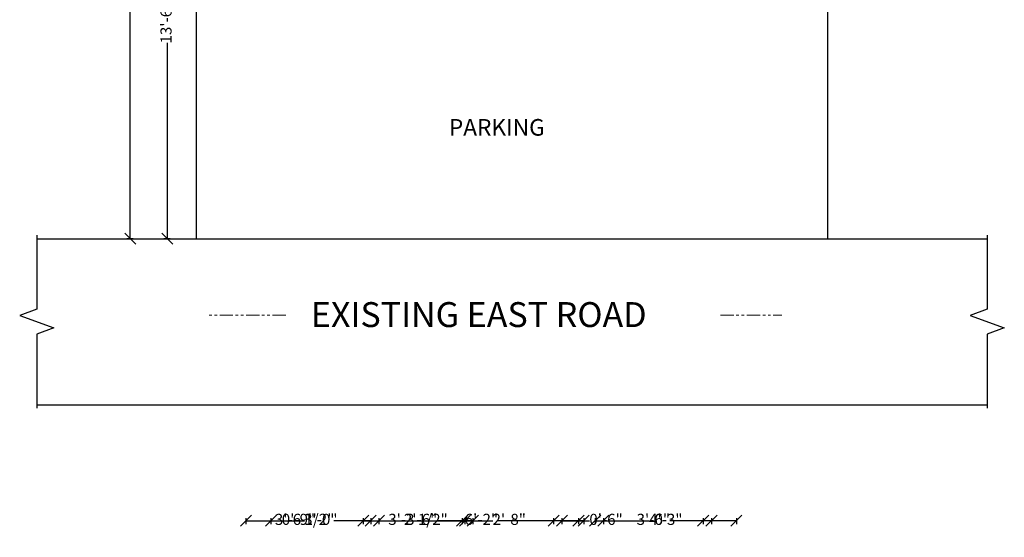
# Model space of a CAD drawing. Units: inches. Extents: x 2349 to 2798, y 397 to 1271.
# Tile 1 of 3: x 2396 to 2751, y 397 to 584. Entities that reach past the tile are written whole.
import ezdxf

# ---------------------------------------------------------------- set-up
doc = ezdxf.new("R2010")
doc.units = ezdxf.units.IN
doc.linetypes.add('PHANTOM2', pattern=[31.75, 15.875, -3.175, 3.175, -3.175, 3.175, -3.175])
for name, color, linetype, lineweight in [('A-ANNO-DIMS', 2, 'Continuous', 18), ('A-ANNO-TEXT', 7, 'Continuous', 18), ('A-AREA-IDEN', 7, 'Continuous', 18), ('C-PROP', 7, 'Continuous', 25), ('C-ROAD', 7, 'Continuous', 25), ('C-ROAD-CNTR', 7, 'PHANTOM2', 13)]:
    doc.layers.add(name, color=color, linetype=linetype, lineweight=lineweight)
doc.styles.get("Standard").update_dxf_attribs({"font": 'arial.ttf'})
doc.dimstyles.new('ISO-25', dxfattribs={"dimtxt": 4, "dimasz": 4, "dimexe": 1.25, "dimexo": 1, "dimtad": 0, "dimdec": 1, "dimlunit": 3, "dimtxsty": 'Standard', "dimblk": 'OBLIQUE', "dimcen": 2.5, "dimclrd": 1, "dimclrt": 3, "dimadec": 0, "dimazin": 0, "dimtfac": 1, "dimtdec": 1, "dimtmove": 0, "dimatfit": 3, "dimfxl": 1, "dimfxlon": 1, "dimarcsym": 0})

# ---------------------------------------------------------------- blocks, each defined once
blk = doc.blocks.new('_Oblique')
at = {"color": 0, "linetype": 'ByBlock', "lineweight": -2}
blk.add_line((-0.5, -0.5), (0.5, 0.5), dxfattribs=at)
blk = doc.blocks.new('*D9')
at = {"layer": 'A-ANNO-DIMS', "color": 0, "lineweight": -2, "transparency": 16777216}
for p, q in [((2450.39, 660.52), (2448.14, 660.52)), ((2449.39, 660.52), (2449.39, 589.82)), ((2449.39, 504.52), (2449.39, 575.21)), ((2450.39, 504.52), (2448.14, 504.52))]:
    blk.add_line(p, q, dxfattribs=at)
at = {"layer": 'Defpoints', "color": 0, "transparency": 16777216}
for p in [(2459.73, 660.52), (2449.39, 504.52), (2459.73, 504.52)]:
    blk.add_point(p, dxfattribs=at)
at = {"layer": 'A-ANNO-DIMS', "color": 0, "lineweight": -2, "transparency": 16777216, "xscale": 4, "yscale": 4, "zscale": 4}
for p, rotation in [((2449.39, 660.52), 90), ((2449.39, 504.52), 270)]:
    blk.add_blockref('_Oblique', p, dxfattribs=dict(at, rotation=rotation))
at = {"layer": 'A-ANNO-DIMS', "color": 0, "transparency": 16777216, "insert": (2449.39, 582.52), "char_height": 4, "attachment_point": 5, "rotation": 90}
blk.add_mtext('13\'-6"', dxfattribs=at)
blk = doc.blocks.new('*D10')
at = {"layer": 'A-ANNO-DIMS', "color": 0, "lineweight": -2, "transparency": 16777216}
for p, q in [((2436.96, 1224.52), (2434.71, 1224.52)), ((2435.96, 1224.52), (2435.96, 868.55)), ((2435.96, 504.52), (2435.96, 860.49)), ((2436.96, 504.52), (2434.71, 504.52))]:
    blk.add_line(p, q, dxfattribs=at)
at = {"layer": 'Defpoints', "color": 0, "transparency": 16777216}
for p in [(2459.73, 1224.52), (2435.96, 504.52), (2459.73, 504.52)]:
    blk.add_point(p, dxfattribs=at)
at = {"layer": 'A-ANNO-DIMS', "color": 0, "lineweight": -2, "transparency": 16777216, "xscale": 4, "yscale": 4, "zscale": 4}
for p, rotation in [((2435.96, 1224.52), 90), ((2435.96, 504.52), 270)]:
    blk.add_blockref('_Oblique', p, dxfattribs=dict(at, rotation=rotation))
at = {"layer": 'A-ANNO-DIMS', "color": 0, "transparency": 16777216, "insert": (2435.96, 864.52), "char_height": 4, "attachment_point": 5, "rotation": 90}
blk.add_mtext("60'", dxfattribs=at)
blk = doc.blocks.new('ROAD-BREAK')
blk.add_lwpolyline([(0, 0), (0, -26.75), (-6.18, -29), (6.18, -33.5), (0, -35.75), (0, -62.5)])
blk = doc.blocks.new('*D28')
at = {"layer": 'A-ANNO-DIMS', "color": 0, "lineweight": -2, "transparency": 16777216}
for p, q in [((2603.73, 403.67), (2603.73, 401.42)), ((2654.73, 403.67), (2654.73, 401.42))]:
    blk.add_line(p, q, dxfattribs=at)
at = {"layer": 'A-ANNO-DIMS', "color": 1, "lineweight": -2, "transparency": 16777216}
for p, q in [((2603.73, 402.67), (2623.21, 402.67)), ((2654.73, 402.67), (2635.25, 402.67))]:
    blk.add_line(p, q, dxfattribs=at)
at = {"layer": 'Defpoints', "color": 0, "transparency": 16777216}
for p in [(2603.73, 660.52), (2654.73, 660.52), (2654.73, 402.67)]:
    blk.add_point(p, dxfattribs=at)
at = {"layer": 'A-ANNO-DIMS', "color": 1, "lineweight": -2, "transparency": 16777216, "xscale": 4, "yscale": 4, "zscale": 4, "rotation": 180}
blk.add_blockref('_Oblique', (2603.73, 402.67), dxfattribs=at)
at = {"layer": 'A-ANNO-DIMS', "color": 1, "lineweight": -2, "transparency": 16777216, "xscale": 4, "yscale": 4, "zscale": 4}
blk.add_blockref('_Oblique', (2654.73, 402.67), dxfattribs=at)
at = {"layer": 'A-ANNO-DIMS', "color": 3, "transparency": 16777216, "insert": (2629.23, 402.67), "char_height": 4, "attachment_point": 5}
blk.add_mtext('4\'-3"', dxfattribs=at)
blk = doc.blocks.new('*D29')
at = {"layer": 'A-ANNO-DIMS', "color": 0, "lineweight": -2, "transparency": 16777216}
for p, q in [((2477.73, 403.67), (2477.73, 401.42)), ((2520.04, 403.67), (2520.04, 401.42))]:
    blk.add_line(p, q, dxfattribs=at)
at = {"layer": 'A-ANNO-DIMS', "color": 1, "lineweight": -2, "transparency": 16777216}
for p, q in [((2477.73, 402.67), (2488.28, 402.67)), ((2520.04, 402.67), (2509.48, 402.67))]:
    blk.add_line(p, q, dxfattribs=at)
at = {"layer": 'Defpoints', "color": 0, "transparency": 16777216}
for p in [(2477.73, 660.52), (2520.04, 660.52), (2520.04, 402.67)]:
    blk.add_point(p, dxfattribs=at)
at = {"layer": 'A-ANNO-DIMS', "color": 1, "lineweight": -2, "transparency": 16777216, "xscale": 4, "yscale": 4, "zscale": 4, "rotation": 180}
blk.add_blockref('_Oblique', (2477.73, 402.67), dxfattribs=at)
at = {"layer": 'A-ANNO-DIMS', "color": 1, "lineweight": -2, "transparency": 16777216, "xscale": 4, "yscale": 4, "zscale": 4}
blk.add_blockref('_Oblique', (2520.04, 402.67), dxfattribs=at)
at = {"layer": 'A-ANNO-DIMS', "color": 3, "transparency": 16777216, "insert": (2498.88, 402.67), "char_height": 4, "attachment_point": 5}
blk.add_mtext('3\'-6 1/2"', dxfattribs=at)
blk = doc.blocks.new('*D30')
at = {"layer": 'A-ANNO-DIMS', "color": 0, "lineweight": -2, "transparency": 16777216}
for p, q in [((2520.04, 403.67), (2520.04, 401.42)), ((2559.59, 403.67), (2559.59, 401.42))]:
    blk.add_line(p, q, dxfattribs=at)
at = {"layer": 'A-ANNO-DIMS', "color": 1, "lineweight": -2, "transparency": 16777216}
for p, q in [((2520.04, 402.67), (2529.21, 402.67)), ((2559.59, 402.67), (2550.42, 402.67))]:
    blk.add_line(p, q, dxfattribs=at)
at = {"layer": 'Defpoints', "color": 0, "transparency": 16777216}
for p in [(2520.04, 660.52), (2559.59, 660.52), (2559.59, 402.67)]:
    blk.add_point(p, dxfattribs=at)
at = {"layer": 'A-ANNO-DIMS', "color": 1, "lineweight": -2, "transparency": 16777216, "xscale": 4, "yscale": 4, "zscale": 4, "rotation": 180}
blk.add_blockref('_Oblique', (2520.04, 402.67), dxfattribs=at)
at = {"layer": 'A-ANNO-DIMS', "color": 1, "lineweight": -2, "transparency": 16777216, "xscale": 4, "yscale": 4, "zscale": 4}
blk.add_blockref('_Oblique', (2559.59, 402.67), dxfattribs=at)
at = {"layer": 'A-ANNO-DIMS', "color": 3, "transparency": 16777216, "insert": (2539.81, 402.67), "char_height": 4, "attachment_point": 5}
blk.add_mtext('3\'-3 1/2"', dxfattribs=at)
blk = doc.blocks.new('*D31')
at = {"layer": 'A-ANNO-DIMS', "color": 0, "lineweight": -2, "transparency": 16777216}
for p, q in [((2603.73, 403.67), (2603.73, 401.42)), ((2645.73, 403.67), (2645.73, 401.42))]:
    blk.add_line(p, q, dxfattribs=at)
at = {"layer": 'A-ANNO-DIMS', "color": 1, "lineweight": -2, "transparency": 16777216}
for p, q in [((2603.73, 402.67), (2618.79, 402.67)), ((2645.73, 402.67), (2630.67, 402.67))]:
    blk.add_line(p, q, dxfattribs=at)
at = {"layer": 'Defpoints', "color": 0, "transparency": 16777216}
for p in [(2603.73, 792.52), (2645.73, 792.52), (2645.73, 402.67)]:
    blk.add_point(p, dxfattribs=at)
at = {"layer": 'A-ANNO-DIMS', "color": 1, "lineweight": -2, "transparency": 16777216, "xscale": 4, "yscale": 4, "zscale": 4, "rotation": 180}
blk.add_blockref('_Oblique', (2603.73, 402.67), dxfattribs=at)
at = {"layer": 'A-ANNO-DIMS', "color": 1, "lineweight": -2, "transparency": 16777216, "xscale": 4, "yscale": 4, "zscale": 4}
blk.add_blockref('_Oblique', (2645.73, 402.67), dxfattribs=at)
at = {"layer": 'A-ANNO-DIMS', "color": 3, "transparency": 16777216, "insert": (2624.73, 402.67), "char_height": 4, "attachment_point": 5}
blk.add_mtext('3\'-6"', dxfattribs=at)
blk = doc.blocks.new('*D32')
at = {"layer": 'A-ANNO-DIMS', "color": 0, "lineweight": -2, "transparency": 16777216}
for p, q in [((2606.73, 403.67), (2606.73, 401.42)), ((2642.73, 403.67), (2642.73, 401.42))]:
    blk.add_line(p, q, dxfattribs=at)
at = {"layer": 'A-ANNO-DIMS', "color": 1, "lineweight": -2, "transparency": 16777216}
for p, q in [((2606.73, 402.67), (2618.79, 402.67)), ((2642.73, 402.67), (2630.67, 402.67))]:
    blk.add_line(p, q, dxfattribs=at)
at = {"layer": 'Defpoints', "color": 0, "transparency": 16777216}
for p in [(2606.73, 981.52), (2642.73, 981.52), (2642.73, 402.67)]:
    blk.add_point(p, dxfattribs=at)
at = {"layer": 'A-ANNO-DIMS', "color": 1, "lineweight": -2, "transparency": 16777216, "xscale": 4, "yscale": 4, "zscale": 4, "rotation": 180}
blk.add_blockref('_Oblique', (2606.73, 402.67), dxfattribs=at)
at = {"layer": 'A-ANNO-DIMS', "color": 1, "lineweight": -2, "transparency": 16777216, "xscale": 4, "yscale": 4, "zscale": 4}
blk.add_blockref('_Oblique', (2642.73, 402.67), dxfattribs=at)
at = {"layer": 'A-ANNO-DIMS', "color": 3, "transparency": 16777216, "insert": (2624.73, 402.67), "char_height": 4, "attachment_point": 5}
blk.add_mtext('3\'-0"', dxfattribs=at)
blk = doc.blocks.new('*D33')
at = {"layer": 'A-ANNO-DIMS', "color": 0, "lineweight": -2, "transparency": 16777216}
for p, q in [((2556.73, 403.67), (2556.73, 401.42)), ((2588.73, 403.67), (2588.73, 401.42))]:
    blk.add_line(p, q, dxfattribs=at)
at = {"layer": 'A-ANNO-DIMS', "color": 1, "lineweight": -2, "transparency": 16777216}
for p, q in [((2556.73, 402.67), (2566.76, 402.67)), ((2588.73, 402.67), (2578.71, 402.67))]:
    blk.add_line(p, q, dxfattribs=at)
at = {"layer": 'Defpoints', "color": 0, "transparency": 16777216}
for p in [(2556.73, 1143.52), (2588.73, 1143.52), (2588.73, 402.67)]:
    blk.add_point(p, dxfattribs=at)
at = {"layer": 'A-ANNO-DIMS', "color": 1, "lineweight": -2, "transparency": 16777216, "xscale": 4, "yscale": 4, "zscale": 4, "rotation": 180}
blk.add_blockref('_Oblique', (2556.73, 402.67), dxfattribs=at)
at = {"layer": 'A-ANNO-DIMS', "color": 1, "lineweight": -2, "transparency": 16777216, "xscale": 4, "yscale": 4, "zscale": 4}
blk.add_blockref('_Oblique', (2588.73, 402.67), dxfattribs=at)
at = {"layer": 'A-ANNO-DIMS', "color": 3, "transparency": 16777216, "insert": (2572.73, 402.67), "char_height": 4, "attachment_point": 5}
blk.add_mtext('2\'-8"', dxfattribs=at)
blk = doc.blocks.new('*D39')
at = {"layer": 'A-ANNO-DIMS', "color": 0, "lineweight": -2, "transparency": 16777216}
for p, q in [((2486.73, 403.67), (2486.73, 401.42)), ((2522.73, 403.67), (2522.73, 401.42))]:
    blk.add_line(p, q, dxfattribs=at)
at = {"layer": 'A-ANNO-DIMS', "color": 1, "lineweight": -2, "transparency": 16777216}
for p, q in [((2486.73, 402.67), (2498.79, 402.67)), ((2522.73, 402.67), (2510.67, 402.67))]:
    blk.add_line(p, q, dxfattribs=at)
at = {"layer": 'Defpoints', "color": 0, "transparency": 16777216}
for p in [(2486.73, 836.92), (2522.73, 836.92), (2522.73, 402.67)]:
    blk.add_point(p, dxfattribs=at)
at = {"layer": 'A-ANNO-DIMS', "color": 1, "lineweight": -2, "transparency": 16777216, "xscale": 4, "yscale": 4, "zscale": 4, "rotation": 180}
blk.add_blockref('_Oblique', (2486.73, 402.67), dxfattribs=at)
at = {"layer": 'A-ANNO-DIMS', "color": 1, "lineweight": -2, "transparency": 16777216, "xscale": 4, "yscale": 4, "zscale": 4}
blk.add_blockref('_Oblique', (2522.73, 402.67), dxfattribs=at)
at = {"layer": 'A-ANNO-DIMS', "color": 3, "transparency": 16777216, "insert": (2504.73, 402.67), "char_height": 4, "attachment_point": 5}
blk.add_mtext('3\'-0"', dxfattribs=at)
blk = doc.blocks.new('*D40')
at = {"layer": 'A-ANNO-DIMS', "color": 0, "lineweight": -2, "transparency": 16777216}
for p, q in [((2525.73, 403.67), (2525.73, 401.42)), ((2555.73, 403.67), (2555.73, 401.42))]:
    blk.add_line(p, q, dxfattribs=at)
at = {"layer": 'A-ANNO-DIMS', "color": 1, "lineweight": -2, "transparency": 16777216}
for p, q in [((2525.73, 402.67), (2534.76, 402.67)), ((2555.73, 402.67), (2546.71, 402.67))]:
    blk.add_line(p, q, dxfattribs=at)
at = {"layer": 'Defpoints', "color": 0, "transparency": 16777216}
for p in [(2555.73, 801.52), (2525.73, 795.52), (2555.73, 402.67)]:
    blk.add_point(p, dxfattribs=at)
at = {"layer": 'A-ANNO-DIMS', "color": 1, "lineweight": -2, "transparency": 16777216, "xscale": 4, "yscale": 4, "zscale": 4, "rotation": 180}
blk.add_blockref('_Oblique', (2525.73, 402.67), dxfattribs=at)
at = {"layer": 'A-ANNO-DIMS', "color": 1, "lineweight": -2, "transparency": 16777216, "xscale": 4, "yscale": 4, "zscale": 4}
blk.add_blockref('_Oblique', (2555.73, 402.67), dxfattribs=at)
at = {"layer": 'A-ANNO-DIMS', "color": 3, "transparency": 16777216, "insert": (2540.73, 402.67), "char_height": 4, "attachment_point": 5}
blk.add_mtext('2\'-6"', dxfattribs=at)
blk = doc.blocks.new('*D46')
at = {"layer": 'A-ANNO-DIMS', "color": 0, "lineweight": -2, "transparency": 16777216}
for p, q in [((2591.73, 403.67), (2591.73, 401.42)), ((2597.73, 403.67), (2597.73, 401.42))]:
    blk.add_line(p, q, dxfattribs=at)
at = {"layer": 'A-ANNO-DIMS', "color": 1, "lineweight": -2, "transparency": 16777216}
for p, q in [((2591.73, 402.67), (2597.73, 402.67)), ((2597.73, 402.67), (2601.73, 402.67))]:
    blk.add_line(p, q, dxfattribs=at)
at = {"layer": 'Defpoints', "color": 0, "transparency": 16777216}
for p in [(2591.73, 1206.52), (2597.73, 1206.52), (2597.73, 402.67)]:
    blk.add_point(p, dxfattribs=at)
at = {"layer": 'A-ANNO-DIMS', "color": 1, "lineweight": -2, "transparency": 16777216, "xscale": 4, "yscale": 4, "zscale": 4, "rotation": 180}
blk.add_blockref('_Oblique', (2591.73, 402.67), dxfattribs=at)
at = {"layer": 'A-ANNO-DIMS', "color": 1, "lineweight": -2, "transparency": 16777216, "xscale": 4, "yscale": 4, "zscale": 4}
blk.add_blockref('_Oblique', (2597.73, 402.67), dxfattribs=at)
at = {"layer": 'A-ANNO-DIMS', "color": 3, "transparency": 16777216, "insert": (2607.67, 402.67), "char_height": 4, "attachment_point": 5}
blk.add_mtext('0\'-6"', dxfattribs=at)
blk = doc.blocks.new('*D47')
at = {"layer": 'A-ANNO-DIMS', "color": 0, "lineweight": -2, "transparency": 16777216}
for p, q in [((2477.73, 403.67), (2477.73, 401.42)), ((2486.73, 403.67), (2486.73, 401.42))]:
    blk.add_line(p, q, dxfattribs=at)
at = {"layer": 'A-ANNO-DIMS', "color": 1, "lineweight": -2, "transparency": 16777216}
for p, q in [((2477.73, 402.67), (2486.73, 402.67)), ((2486.73, 402.67), (2490.73, 402.67))]:
    blk.add_line(p, q, dxfattribs=at)
at = {"layer": 'Defpoints', "color": 0, "transparency": 16777216}
for p in [(2477.73, 1212.52), (2486.73, 1206.52), (2486.73, 402.67)]:
    blk.add_point(p, dxfattribs=at)
at = {"layer": 'A-ANNO-DIMS', "color": 1, "lineweight": -2, "transparency": 16777216, "xscale": 4, "yscale": 4, "zscale": 4, "rotation": 180}
blk.add_blockref('_Oblique', (2477.73, 402.67), dxfattribs=at)
at = {"layer": 'A-ANNO-DIMS', "color": 1, "lineweight": -2, "transparency": 16777216, "xscale": 4, "yscale": 4, "zscale": 4}
blk.add_blockref('_Oblique', (2486.73, 402.67), dxfattribs=at)
at = {"layer": 'A-ANNO-DIMS', "color": 3, "transparency": 16777216, "insert": (2496.67, 402.67), "char_height": 4, "attachment_point": 5}
blk.add_mtext('0\'-9"', dxfattribs=at)
blk = doc.blocks.new('*D48')
at = {"layer": 'A-ANNO-DIMS', "color": 0, "lineweight": -2, "transparency": 16777216}
for p, q in [((2525.73, 403.67), (2525.73, 401.42)), ((2599.63, 403.67), (2599.63, 401.42))]:
    blk.add_line(p, q, dxfattribs=at)
at = {"layer": 'A-ANNO-DIMS', "color": 1, "lineweight": -2, "transparency": 16777216}
for p, q in [((2525.73, 402.67), (2556.73, 402.67)), ((2599.63, 402.67), (2568.63, 402.67))]:
    blk.add_line(p, q, dxfattribs=at)
at = {"layer": 'Defpoints', "color": 0, "transparency": 16777216}
for p in [(2525.73, 942.52), (2599.63, 942.52), (2599.63, 402.67)]:
    blk.add_point(p, dxfattribs=at)
at = {"layer": 'A-ANNO-DIMS', "color": 1, "lineweight": -2, "transparency": 16777216, "xscale": 4, "yscale": 4, "zscale": 4, "rotation": 180}
blk.add_blockref('_Oblique', (2525.73, 402.67), dxfattribs=at)
at = {"layer": 'A-ANNO-DIMS', "color": 1, "lineweight": -2, "transparency": 16777216, "xscale": 4, "yscale": 4, "zscale": 4}
blk.add_blockref('_Oblique', (2599.63, 402.67), dxfattribs=at)
at = {"layer": 'A-ANNO-DIMS', "color": 3, "transparency": 16777216, "insert": (2562.68, 402.67), "char_height": 4, "attachment_point": 5}
blk.add_mtext('6\'-2"', dxfattribs=at)

msp = doc.modelspace()

# ---------------------------------------------------------------- linework, layer by layer
at = {"layer": 'C-PROP'}
for p, q in [((2459.73, 1224.52), (2459.73, 504.52)), ((2687.73, 504.52), (2687.73, 1224.52))]:
    msp.add_line(p, q, dxfattribs=at)
at = {"layer": 'C-ROAD'}
for p, q in [((2402.25, 504.52), (2745.21, 504.52)), ((2402.25, 444.52), (2745.21, 444.52))]:
    msp.add_line(p, q, dxfattribs=at)
at = {"layer": 'C-ROAD-CNTR', "ltscale": 0.3}
for p, q in [((2492.08, 476.9), (2464.15, 476.9)), ((2648.97, 476.9), (2671.08, 476.9))]:
    msp.add_line(p, q, dxfattribs=at)

# ---------------------------------------------------------------- block references
at = {"layer": 'C-ROAD'}
for p in [(2402.25, 505.77), (2745.21, 505.77)]:
    msp.add_blockref('ROAD-BREAK', p, dxfattribs=at)

# ---------------------------------------------------------------- texts
at = {"layer": 'A-ANNO-TEXT', "insert": (2501.16, 481.61), "char_height": 9, "attachment_point": 1}
msp.add_mtext_dynamic_manual_height_columns('EXISTING EAST ROAD', width=143.1143, gutter_width=12.5, heights=[0], dxfattribs=at)
at = {"layer": 'A-AREA-IDEN', "insert": (2526.9, 547.71), "char_height": 6, "attachment_point": 1}
msp.add_mtext_dynamic_manual_height_columns('\\pxqc;PARKING', width=82.6982, gutter_width=12.5, heights=[0], dxfattribs=at)

# ---------------------------------------------------------------- dimensions: what is measured, and where the dimension line sits
at = {"layer": 'A-ANNO-DIMS'}
dim = msp.add_linear_dim(base=(2435.96, 504.52), p1=(2459.73, 1224.52), p2=(2459.73, 504.52), angle=90, dimstyle='ISO-25', override={"dimclrd": 0, "dimclre": 0, "dimclrt": 0}, dxfattribs=at)
dim.commit()
dim.dimension.update_dxf_attribs({"geometry": '*D10', "text_midpoint": (2435.96, 864.52)})
for base, p1, p2, picture, middle in [((2486.73, 402.67), (2477.73, 1212.52), (2486.73, 1206.52), '*D47', (2496.67, 402.67)), ((2597.73, 402.67), (2591.73, 1206.52), (2597.73, 1206.52), '*D46', (2607.67, 402.67)), ((2588.73, 402.67), (2556.73, 1143.52), (2588.73, 1143.52), '*D33', (2572.73, 402.67)), ((2642.73, 402.67), (2606.73, 981.52), (2642.73, 981.52), '*D32', (2624.73, 402.67)), ((2599.63, 402.67), (2525.73, 942.52), (2599.63, 942.52), '*D48', (2562.68, 402.67)), ((2522.73, 402.67), (2486.73, 836.92), (2522.73, 836.92), '*D39', (2504.73, 402.67)), ((2555.73, 402.67), (2525.73, 795.52), (2555.73, 801.52), '*D40', (2540.73, 402.67)), ((2645.73, 402.67), (2603.73, 792.52), (2645.73, 792.52), '*D31', (2624.73, 402.67)), ((2520.04, 402.67), (2477.73, 660.52), (2520.04, 660.52), '*D29', (2498.88, 402.67)), ((2559.5941, 402.6665), (2520.0358, 660.5165), (2559.5941, 660.5165), '*D30', (2539.8149, 402.6665)), ((2654.73, 402.67), (2603.73, 660.52), (2654.73, 660.52), '*D28', (2629.23, 402.67))]:
    dim = msp.add_linear_dim(base=base, p1=p1, p2=p2, dimstyle='ISO-25', override={"dimdec": 1, "dimlfac": 1, "dimrnd": 0, "dimzin": 1, "dimdsep": 46, "dimlunit": 4, "dimfrac": 2}, dxfattribs=at)
    dim.commit()
    dim.dimension.update_dxf_attribs({"geometry": picture, "text_midpoint": middle})
dim = msp.add_linear_dim(base=(2449.39, 504.52), p1=(2459.73, 660.52), p2=(2459.73, 504.52), angle=90, text='13\'-6"', dimstyle='ISO-25', override={"dimclrd": 0, "dimclre": 0, "dimclrt": 0, "dimtmove": 1}, dxfattribs=at)
dim.commit()
dim.dimension.update_dxf_attribs({"geometry": '*D9', "text_midpoint": (2449.39, 582.52)})

doc.saveas('drawing.dxf')
